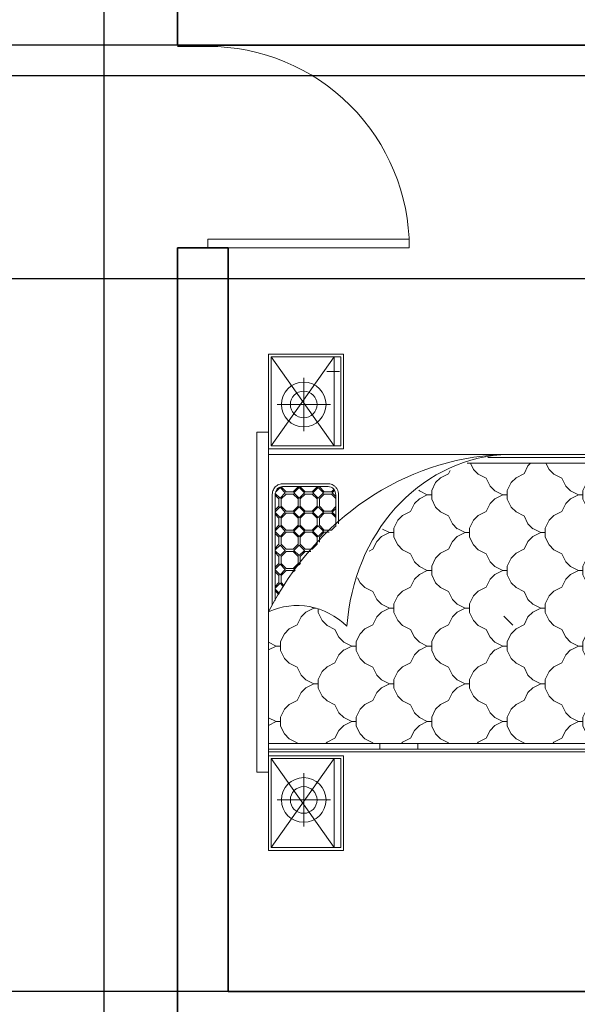
# Model space of a CAD drawing. Units: inches. Extents: x 1624 to 3956, y 1589 to 5028.
# Tile 4 of 16: x 1915 to 2014, y 2075 to 2250. Entities that reach past the tile are written whole.
import ezdxf

# ---------------------------------------------------------------- set-up
doc = ezdxf.new("R2010")
doc.units = ezdxf.units.IN
for name, color, linetype, lineweight in [('A-ANNO-DIMS', 2, 'Continuous', 13), ('A-DOOR', 3, 'Continuous', 18), ('A-FURN', 8, 'Continuous', 18), ('A-WALL', 7, 'Continuous', 35)]:
    doc.layers.add(name, color=color, linetype=linetype, lineweight=lineweight)
doc.styles.get("Standard").update_dxf_attribs({"font": 'arial.ttf'})
doc.dimstyles.new('Copy of ISO-25', dxfattribs={"dimtxt": 2.5, "dimasz": 2.5, "dimexe": 1.25, "dimexo": 0.625, "dimtad": 1, "dimdec": 1, "dimlunit": 4, "dimtxsty": 'Standard', "dimcen": 2.5, "dimadec": 0, "dimazin": 0, "dimtfac": 1, "dimtdec": 1, "dimtmove": 0, "dimatfit": 3, "dimfxl": 1, "dimarcsym": 0})

# ---------------------------------------------------------------- blocks, each defined once
blk = doc.blocks.new('*U5')
for p, q in [((0, 0), (0, 6)), ((40, 0), (40, 6))]:
    blk.add_line(p, q)
blk.add_lwpolyline([(0, 0), (0, -40), (1.75, -40), (1.75, 0)], close=True)
blk.add_arc((0, 0), 40, 270, 0)
blk = doc.blocks.new('A$C029D5C69')
for p, q in [((0.4164, 2.0693), (0.4164, 2.0066)), ((2.2315, 2.0693), (0.4164, 2.0693)), ((2.2315, 2.0066), (2.2315, 2.0693)), ((0, 1.606), (0, 2.0066)), ((0, 2.0066), (0.505, 2.0066)), ((0.4164, 2.0066), (2.2315, 2.0066)), ((0.505, 2.0066), (0.505, 1.606)), ((0.5252, 0.0351), (0.5252, 2.0066)), ((0.5403, 0.0502), (0.5403, 2.0066)), ((0.5706, 0.0805), (0.5706, 2.0066)), ((0.6869, 1.966), (0.6666, 2.0066)), ((0.7072, 2.0066), (0.6869, 1.966)), ((1.0902, 1.966), (1.0699, 2.0066)), ((1.1106, 2.0066), (1.0902, 1.966)), ((2.1114, 2.0087), (2.1114, 0.0351)), ((2.6479, 2.0066), (2.1429, 2.0066)), ((2.1429, 2.0066), (2.1429, 1.606)), ((2.6479, 1.606), (2.6479, 2.0066)), ((0.0151, 1.6211), (0.0151, 1.9915)), ((0.0151, 1.9915), (0.4899, 1.9915)), ((0.2689, 1.9609), (0.2689, 1.6764)), ((0.4899, 1.9915), (0.4899, 1.6211)), ((0.6869, 1.9425), (0.6869, 1.966)), ((0.6869, 1.9425), (0.6869, 1.966)), ((1.0902, 1.9425), (1.0902, 1.966)), ((1.0902, 1.9425), (1.0902, 1.966)), ((1.8954, 1.9865), (1.3081, 1.9865)), ((1.8954, 1.9713), (1.3339, 1.9713)), ((1.3849, 1.9713), (1.3656, 1.952)), ((1.3945, 1.9713), (1.3714, 1.9483)), ((1.4249, 1.945), (1.3986, 1.9713)), ((1.4249, 1.945), (1.4059, 1.926)), ((1.4288, 1.9507), (1.4081, 1.9713)), ((1.4476, 1.9507), (1.4288, 1.9507)), ((1.4476, 1.9507), (1.4664, 1.9507)), ((1.487, 1.9713), (1.4664, 1.9507)), ((1.4966, 1.9713), (1.4703, 1.945)), ((1.4986, 1.9167), (1.4703, 1.945)), ((1.527, 1.945), (1.4986, 1.9167)), ((1.527, 1.945), (1.5007, 1.9713)), ((1.5309, 1.9507), (1.5102, 1.9713)), ((1.5497, 1.9507), (1.5309, 1.9507)), ((1.5497, 1.9507), (1.5685, 1.9507)), ((1.5891, 1.9713), (1.5685, 1.9507)), ((1.5987, 1.9713), (1.5724, 1.945)), ((1.6007, 1.9167), (1.5724, 1.945)), ((1.6291, 1.945), (1.6007, 1.9167)), ((1.6291, 1.945), (1.6028, 1.9713)), ((1.633, 1.9507), (1.6123, 1.9713)), ((1.6518, 1.9507), (1.633, 1.9507)), ((1.6518, 1.9507), (1.6706, 1.9507)), ((1.6912, 1.9713), (1.6706, 1.9507)), ((1.7008, 1.9713), (1.6745, 1.945)), ((1.7028, 1.9167), (1.6745, 1.945)), ((1.7312, 1.945), (1.7028, 1.9167)), ((1.7312, 1.945), (1.7049, 1.9713)), ((1.7351, 1.9507), (1.7144, 1.9713)), ((1.7539, 1.9507), (1.7351, 1.9507)), ((1.7539, 1.9507), (1.7727, 1.9507)), ((1.7933, 1.9713), (1.7727, 1.9507)), ((1.8029, 1.9713), (1.7766, 1.945)), ((1.8049, 1.9167), (1.7766, 1.945)), ((1.8333, 1.945), (1.8049, 1.9167)), ((1.8333, 1.945), (1.807, 1.9713)), ((1.8372, 1.9507), (1.8165, 1.9713)), ((1.856, 1.9507), (1.8372, 1.9507)), ((1.856, 1.9507), (1.8748, 1.9507)), ((1.8954, 1.9713), (1.8748, 1.9507)), ((1.9043, 1.9707), (1.8787, 1.945)), ((1.907, 1.9167), (1.8787, 1.945)), ((1.9354, 1.945), (1.907, 1.9167)), ((1.9354, 1.945), (1.9114, 1.969)), ((2.6328, 1.9915), (2.158, 1.9915)), ((2.158, 1.9915), (2.158, 1.6211)), ((2.379, 1.9609), (2.379, 1.6764)), ((2.6328, 1.6211), (2.6328, 1.9915)), ((0.5955, 1.8958), (0.5743, 1.8534)), ((0.621, 1.9213), (0.5955, 1.8958)), ((0.6634, 1.9425), (0.621, 1.9213)), ((0.6634, 1.9425), (0.621, 1.9213)), ((0.6869, 1.9425), (0.6634, 1.9425)), ((0.6869, 1.9425), (0.7104, 1.9425)), ((0.7528, 1.9213), (0.7104, 1.9425)), ((0.7528, 1.9213), (0.7104, 1.9425)), ((0.7783, 1.8958), (0.7528, 1.9213)), ((0.7995, 1.8534), (0.7783, 1.8958)), ((0.9989, 1.8958), (0.9777, 1.8534)), ((1.0243, 1.9213), (0.9988, 1.8958)), ((1.0668, 1.9425), (1.0244, 1.9213)), ((1.0668, 1.9425), (1.0244, 1.9213)), ((1.0902, 1.9425), (1.0668, 1.9425)), ((1.0902, 1.9425), (1.1137, 1.9425)), ((1.1561, 1.9213), (1.1137, 1.9425)), ((1.1561, 1.9213), (1.1137, 1.9425)), ((1.1816, 1.8958), (1.1561, 1.9213)), ((1.2028, 1.8534), (1.1816, 1.8958)), ((1.4288, 1.9394), (1.4116, 1.9222)), ((1.4288, 1.9393), (1.4476, 1.9393)), ((1.4664, 1.9393), (1.4476, 1.9393)), ((1.493, 1.9128), (1.4664, 1.9394)), ((1.493, 1.8752), (1.493, 1.9128)), ((1.5309, 1.9394), (1.5043, 1.9128)), ((1.5043, 1.8752), (1.5043, 1.9128)), ((1.5309, 1.9393), (1.5497, 1.9393)), ((1.5685, 1.9393), (1.5497, 1.9393)), ((1.595, 1.9128), (1.5685, 1.9394)), ((1.595, 1.8752), (1.595, 1.9128)), ((1.633, 1.9394), (1.6064, 1.9128)), ((1.6064, 1.8752), (1.6064, 1.9128)), ((1.633, 1.9393), (1.6518, 1.9393)), ((1.6706, 1.9393), (1.6518, 1.9393)), ((1.6971, 1.9128), (1.6706, 1.9394)), ((1.6971, 1.8752), (1.6971, 1.9128)), ((1.7351, 1.9394), (1.7085, 1.9128)), ((1.7085, 1.8752), (1.7085, 1.9128)), ((1.7351, 1.9393), (1.7539, 1.9393)), ((1.7727, 1.9393), (1.7539, 1.9393)), ((1.7992, 1.9128), (1.7727, 1.9394)), ((1.7992, 1.8752), (1.7992, 1.9128)), ((1.8372, 1.9394), (1.8106, 1.9128)), ((1.8106, 1.8752), (1.8106, 1.9128)), ((1.8372, 1.9393), (1.856, 1.9393)), ((1.8748, 1.9393), (1.856, 1.9393)), ((1.9013, 1.9128), (1.8748, 1.9394)), ((1.9013, 1.8752), (1.9013, 1.9128)), ((1.9393, 1.9394), (1.9127, 1.9128)), ((1.9127, 1.8752), (1.9127, 1.9128)), ((1.9393, 1.9393), (1.9404, 1.9393)), ((1.9414, 1.688), (1.9414, 1.931)), ((1.9565, 1.688), (1.9565, 1.931)), ((0.5743, 1.8534), (0.5706, 1.8515)), ((0.5743, 1.8534), (0.5706, 1.8515)), ((0.8419, 1.8322), (0.7995, 1.8534)), ((0.8419, 1.8322), (0.7995, 1.8534)), ((0.9777, 1.8534), (0.9353, 1.8322)), ((0.9777, 1.8534), (0.9353, 1.8322)), ((1.2452, 1.8322), (1.2028, 1.8534)), ((1.2452, 1.8322), (1.2028, 1.8534)), ((1.493, 1.8752), (1.4867, 1.869)), ((1.4986, 1.8713), (1.4922, 1.8648)), ((1.527, 1.8429), (1.4986, 1.8713)), ((1.5309, 1.8486), (1.5043, 1.8752)), ((1.527, 1.8429), (1.5242, 1.8401)), ((1.5497, 1.8486), (1.5309, 1.8486)), ((1.5497, 1.8486), (1.5685, 1.8486)), ((1.595, 1.8752), (1.5685, 1.8486)), ((1.6007, 1.8713), (1.5724, 1.8429)), ((1.6007, 1.8146), (1.5724, 1.8429)), ((1.6291, 1.8429), (1.6007, 1.8713)), ((1.6291, 1.8429), (1.6007, 1.8146)), ((1.633, 1.8486), (1.6064, 1.8752)), ((1.6518, 1.8486), (1.633, 1.8486)), ((1.6518, 1.8486), (1.6706, 1.8486)), ((1.6971, 1.8752), (1.6706, 1.8486)), ((1.7028, 1.8713), (1.6745, 1.8429)), ((1.7028, 1.8146), (1.6745, 1.8429)), ((1.7312, 1.8429), (1.7028, 1.8713)), ((1.7312, 1.8429), (1.7028, 1.8146)), ((1.7351, 1.8486), (1.7085, 1.8752)), ((1.7539, 1.8486), (1.7351, 1.8486)), ((1.7539, 1.8486), (1.7727, 1.8486)), ((1.7992, 1.8752), (1.7727, 1.8486)), ((1.8049, 1.8713), (1.7766, 1.8429)), ((1.8049, 1.8146), (1.7766, 1.8429)), ((1.8333, 1.8429), (1.8049, 1.8713)), ((1.8333, 1.8429), (1.8049, 1.8146)), ((1.8372, 1.8486), (1.8106, 1.8752)), ((1.856, 1.8486), (1.8372, 1.8486)), ((1.856, 1.8486), (1.8748, 1.8486)), ((1.9013, 1.8752), (1.8748, 1.8486)), ((1.907, 1.8713), (1.8787, 1.8429)), ((1.907, 1.8146), (1.8787, 1.8429)), ((1.9354, 1.8429), (1.907, 1.8713)), ((1.9354, 1.8429), (1.907, 1.8146)), ((1.9393, 1.8486), (1.9127, 1.8752)), ((1.9414, 1.8486), (1.9393, 1.8486)), ((0.1267, 1.8186), (0.4111, 1.8186)), ((0.8674, 1.8067), (0.8419, 1.8322)), ((0.8886, 1.7643), (0.8674, 1.8067)), ((0.9098, 1.8067), (0.8886, 1.7643)), ((0.9352, 1.8322), (0.9097, 1.8067)), ((1.2707, 1.8067), (1.2452, 1.8322)), ((1.2919, 1.7643), (1.2707, 1.8067)), ((1.5309, 1.8373), (1.5295, 1.8359)), ((1.5309, 1.8373), (1.5497, 1.8373)), ((1.5685, 1.8373), (1.5497, 1.8373)), ((1.595, 1.8107), (1.5685, 1.8373)), ((1.595, 1.7806), (1.595, 1.8107)), ((1.633, 1.8373), (1.6064, 1.8107)), ((1.6064, 1.7731), (1.6064, 1.8107)), ((1.633, 1.8373), (1.6518, 1.8373)), ((1.6706, 1.8373), (1.6518, 1.8373)), ((1.6971, 1.8107), (1.6706, 1.8373)), ((1.6971, 1.7731), (1.6971, 1.8107)), ((1.7351, 1.8373), (1.7085, 1.8107)), ((1.7085, 1.7731), (1.7085, 1.8107)), ((1.7351, 1.8373), (1.7539, 1.8373)), ((1.7727, 1.8373), (1.7539, 1.8373)), ((1.7992, 1.8107), (1.7727, 1.8373)), ((1.7992, 1.7731), (1.7992, 1.8107)), ((1.8372, 1.8373), (1.8106, 1.8107)), ((1.8106, 1.7731), (1.8106, 1.8107)), ((1.8372, 1.8373), (1.856, 1.8373)), ((1.8748, 1.8373), (1.856, 1.8373)), ((1.9013, 1.8107), (1.8748, 1.8373)), ((1.9013, 1.7731), (1.9013, 1.8107)), ((1.9393, 1.8373), (1.9127, 1.8107)), ((1.9127, 1.7731), (1.9127, 1.8107)), ((1.9393, 1.8373), (1.9414, 1.8373)), ((2.2367, 1.8186), (2.5212, 1.8186)), ((0.8651, 1.7408), (0.8227, 1.7196)), ((0.8651, 1.7408), (0.8227, 1.7196)), ((0.912, 1.7408), (0.8651, 1.7408)), ((0.8886, 1.7408), (0.8886, 1.7643)), ((0.9544, 1.7196), (0.912, 1.7408)), ((0.9544, 1.7196), (0.912, 1.7408)), ((1.2684, 1.7408), (1.226, 1.7196)), ((1.2684, 1.7408), (1.226, 1.7196)), ((1.2885, 1.7408), (1.2684, 1.7408)), ((1.2981, 1.7768), (1.2919, 1.7643)), ((1.2919, 1.7519), (1.2919, 1.7643)), ((1.633, 1.7465), (1.6064, 1.7731)), ((1.6518, 1.7465), (1.633, 1.7465)), ((1.6443, 1.7352), (1.6518, 1.7352)), ((1.6518, 1.7465), (1.6706, 1.7465)), ((1.6706, 1.7352), (1.6518, 1.7352)), ((1.6971, 1.7731), (1.6706, 1.7465)), ((1.6971, 1.7086), (1.6706, 1.7352)), ((1.7028, 1.7692), (1.6745, 1.7408)), ((1.7028, 1.7125), (1.6745, 1.7408)), ((1.7312, 1.7408), (1.7028, 1.7692)), ((1.7312, 1.7408), (1.7028, 1.7125)), ((1.7351, 1.7465), (1.7085, 1.7731)), ((1.7351, 1.7352), (1.7085, 1.7086)), ((1.7539, 1.7465), (1.7351, 1.7465)), ((1.7351, 1.7352), (1.7539, 1.7352)), ((1.7539, 1.7465), (1.7727, 1.7465)), ((1.7727, 1.7352), (1.7539, 1.7352)), ((1.7992, 1.7731), (1.7727, 1.7465)), ((1.7992, 1.7086), (1.7727, 1.7352)), ((1.8049, 1.7692), (1.7766, 1.7408)), ((1.8049, 1.7125), (1.7766, 1.7408)), ((1.8333, 1.7408), (1.8049, 1.7692)), ((1.8333, 1.7408), (1.8049, 1.7125)), ((1.8372, 1.7465), (1.8106, 1.7731)), ((1.8372, 1.7352), (1.8106, 1.7086)), ((1.856, 1.7465), (1.8372, 1.7465)), ((1.8372, 1.7352), (1.856, 1.7352)), ((1.856, 1.7465), (1.8748, 1.7465)), ((1.8748, 1.7352), (1.856, 1.7352)), ((1.9013, 1.7731), (1.8748, 1.7465)), ((1.9013, 1.7086), (1.8748, 1.7352)), ((1.907, 1.7692), (1.8787, 1.7408)), ((1.907, 1.7125), (1.8787, 1.7408)), ((1.9354, 1.7408), (1.907, 1.7692)), ((1.9354, 1.7408), (1.907, 1.7125)), ((1.9393, 1.7465), (1.9127, 1.7731)), ((1.9393, 1.7352), (1.9127, 1.7086)), ((1.9414, 1.7465), (1.9393, 1.7465)), ((1.9393, 1.7352), (1.9414, 1.7352)), ((0.5766, 1.6941), (0.5706, 1.7002)), ((0.5978, 1.6517), (0.5766, 1.6941)), ((0.7972, 1.6941), (0.776, 1.6517)), ((0.8227, 1.7196), (0.7972, 1.6941)), ((0.98, 1.6941), (0.9545, 1.7196)), ((1.0011, 1.6517), (0.9799, 1.6941)), ((1.2005, 1.6941), (1.1793, 1.6517)), ((1.226, 1.7196), (1.2005, 1.6941)), ((1.6971, 1.682), (1.6971, 1.7086)), ((1.7085, 1.671), (1.7085, 1.7086)), ((1.7992, 1.671), (1.7992, 1.7086)), ((1.8106, 1.671), (1.8106, 1.7086)), ((1.9013, 1.671), (1.9013, 1.7086)), ((1.9127, 1.671), (1.9127, 1.7086)), ((2.5551, 1.6275), (2.5551, 1.696)), ((0.6402, 1.6305), (0.5978, 1.6517)), ((0.6402, 1.6305), (0.5978, 1.6517)), ((0.6657, 1.605), (0.6402, 1.6305)), ((0.7336, 1.6305), (0.7081, 1.605)), ((0.776, 1.6517), (0.7336, 1.6305)), ((0.776, 1.6517), (0.7336, 1.6305)), ((1.0435, 1.6305), (1.0011, 1.6517)), ((1.0435, 1.6305), (1.0011, 1.6517)), ((1.0691, 1.605), (1.0436, 1.6305)), ((1.1369, 1.6305), (1.1114, 1.605)), ((1.1793, 1.6517), (1.1369, 1.6305)), ((1.1793, 1.6517), (1.1369, 1.6305)), ((1.7318, 1.6477), (1.7085, 1.671)), ((1.8961, 1.6477), (1.7289, 1.6477)), ((1.8961, 1.6325), (1.7422, 1.6325)), ((1.7992, 1.671), (1.7759, 1.6477)), ((1.8049, 1.6671), (1.7855, 1.6477)), ((1.8244, 1.6477), (1.8049, 1.6671)), ((1.8339, 1.6477), (1.8106, 1.671)), ((1.9013, 1.671), (1.878, 1.6477)), ((1.907, 1.6671), (1.8876, 1.6477)), ((1.9202, 1.6539), (1.907, 1.6671)), ((1.926, 1.6577), (1.9127, 1.671)), ((0.505, 1.606), (0, 1.606)), ((0.4899, 1.6211), (0.0151, 1.6211)), ((0.6869, 1.5626), (0.6657, 1.605)), ((0.7081, 1.605), (0.6869, 1.5626)), ((1.0902, 1.5626), (1.069, 1.605)), ((1.1114, 1.605), (1.0902, 1.5626)), ((2.1429, 1.606), (2.6479, 1.606)), ((2.158, 1.6211), (2.6328, 1.6211)), ((0.6634, 1.5391), (0.621, 1.5179)), ((0.6634, 1.5391), (0.621, 1.5179)), ((0.6869, 1.5392), (0.6634, 1.5392)), ((0.6869, 1.5392), (0.6869, 1.5626)), ((0.6869, 1.5392), (0.6869, 1.5626)), ((0.6869, 1.5392), (0.7104, 1.5392)), ((0.7528, 1.5179), (0.7104, 1.5391)), ((0.7528, 1.5179), (0.7104, 1.5391)), ((1.0668, 1.5391), (1.0244, 1.5179)), ((1.0668, 1.5391), (1.0244, 1.5179)), ((1.0902, 1.5392), (1.0668, 1.5392)), ((1.0902, 1.5392), (1.0902, 1.5626)), ((1.0902, 1.5392), (1.0902, 1.5626)), ((1.0902, 1.5392), (1.1137, 1.5392)), ((1.1561, 1.5179), (1.1137, 1.5391)), ((1.1561, 1.5179), (1.1137, 1.5391)), ((1.4534, 1.5308), (1.4277, 1.5179)), ((1.4534, 1.5308), (1.4277, 1.5179)), ((0.5955, 1.4925), (0.5743, 1.4501)), ((0.621, 1.5179), (0.5955, 1.4924)), ((0.7783, 1.4924), (0.7528, 1.5179)), ((0.7995, 1.4501), (0.7783, 1.4925)), ((0.9989, 1.4925), (0.9777, 1.4501)), ((1.0243, 1.5179), (0.9988, 1.4924)), ((1.1816, 1.4924), (1.1561, 1.5179)), ((1.2028, 1.4501), (1.1816, 1.4925)), ((1.4022, 1.4925), (1.381, 1.4501)), ((1.4277, 1.5179), (1.4022, 1.4924)), ((0.5743, 1.45), (0.5706, 1.4481)), ((0.5743, 1.45), (0.5706, 1.4481)), ((0.8419, 1.4288), (0.7995, 1.45)), ((0.8419, 1.4288), (0.7995, 1.45)), ((0.8674, 1.4033), (0.8419, 1.4288)), ((0.9352, 1.4288), (0.9097, 1.4033)), ((0.9777, 1.45), (0.9353, 1.4288)), ((0.9777, 1.45), (0.9353, 1.4288)), ((1.2452, 1.4288), (1.2028, 1.45)), ((1.2452, 1.4288), (1.2028, 1.45)), ((1.2707, 1.4033), (1.2452, 1.4288)), ((1.3386, 1.4288), (1.3131, 1.4033)), ((1.381, 1.45), (1.3386, 1.4288)), ((1.381, 1.45), (1.3386, 1.4288)), ((1.6062, 1.4501), (1.5966, 1.4692)), ((1.6486, 1.4288), (1.6062, 1.45)), ((1.6486, 1.4288), (1.6062, 1.45)), ((1.6741, 1.4033), (1.6486, 1.4288)), ((0.5403, 1.4117), (0.5706, 1.4117)), ((0.8886, 1.361), (0.8674, 1.4034)), ((0.9098, 1.4034), (0.8886, 1.361)), ((1.2919, 1.361), (1.2707, 1.4034)), ((1.3131, 1.4034), (1.2919, 1.361)), ((1.6953, 1.361), (1.6741, 1.4034)), ((1.714, 1.3984), (1.6953, 1.361)), ((0.8227, 1.3163), (0.7972, 1.2908)), ((0.8651, 1.3374), (0.8227, 1.3162)), ((0.8651, 1.3374), (0.8227, 1.3162)), ((0.912, 1.3375), (0.8651, 1.3375)), ((0.8886, 1.3375), (0.8886, 1.3609)), ((0.9544, 1.3162), (0.912, 1.3374)), ((0.9544, 1.3162), (0.912, 1.3374)), ((0.98, 1.2908), (0.9545, 1.3163)), ((1.226, 1.3163), (1.2005, 1.2908)), ((1.2684, 1.3374), (1.226, 1.3162)), ((1.2684, 1.3374), (1.226, 1.3162)), ((1.3154, 1.3375), (1.2684, 1.3375)), ((1.2919, 1.3375), (1.2919, 1.3609)), ((1.3578, 1.3162), (1.3154, 1.3374)), ((1.3578, 1.3162), (1.3154, 1.3374)), ((1.3833, 1.2908), (1.3578, 1.3163)), ((1.6294, 1.3163), (1.6039, 1.2908)), ((1.6718, 1.3374), (1.6294, 1.3162)), ((1.6718, 1.3374), (1.6294, 1.3162)), ((1.7187, 1.3375), (1.6718, 1.3375)), ((1.6953, 1.3375), (1.6953, 1.3609)), ((1.7611, 1.3162), (1.7187, 1.3374)), ((1.7611, 1.3162), (1.7187, 1.3374)), ((1.7867, 1.2908), (1.7611, 1.3163)), ((0.5766, 1.2908), (0.5706, 1.2968)), ((0.5978, 1.2484), (0.5766, 1.2908)), ((0.7972, 1.2908), (0.776, 1.2484)), ((1.0011, 1.2484), (0.9799, 1.2908)), ((1.2005, 1.2908), (1.1793, 1.2484)), ((1.4045, 1.2484), (1.3833, 1.2908)), ((1.6039, 1.2908), (1.5827, 1.2484)), ((1.8078, 1.2484), (1.7866, 1.2908)), ((0.5403, 1.21), (0.5706, 1.21)), ((0.6402, 1.2271), (0.5978, 1.2483)), ((0.6402, 1.2271), (0.5978, 1.2483)), ((0.6657, 1.2017), (0.6402, 1.2272)), ((0.7336, 1.2272), (0.7081, 1.2017)), ((0.776, 1.2483), (0.7336, 1.2271)), ((0.776, 1.2483), (0.7336, 1.2271)), ((1.0435, 1.2271), (1.0011, 1.2483)), ((1.0435, 1.2271), (1.0011, 1.2483)), ((1.0691, 1.2017), (1.0436, 1.2272)), ((1.1369, 1.2272), (1.1114, 1.2017)), ((1.1793, 1.2483), (1.1369, 1.2271)), ((1.1793, 1.2483), (1.1369, 1.2271)), ((1.4469, 1.2271), (1.4045, 1.2483)), ((1.4469, 1.2271), (1.4045, 1.2483)), ((1.4724, 1.2017), (1.4469, 1.2272)), ((1.5403, 1.2272), (1.5148, 1.2017)), ((1.5827, 1.2483), (1.5403, 1.2271)), ((1.5827, 1.2483), (1.5403, 1.2271)), ((1.8502, 1.2271), (1.8078, 1.2483)), ((1.8502, 1.2271), (1.8078, 1.2483)), ((1.8758, 1.2017), (1.8503, 1.2272)), ((0.6869, 1.1593), (0.6657, 1.2017)), ((0.7081, 1.2017), (0.6869, 1.1593)), ((0.6869, 1.1358), (0.6869, 1.1593)), ((0.6869, 1.1358), (0.6869, 1.1593)), ((1.0902, 1.1593), (1.069, 1.2017)), ((1.1114, 1.2017), (1.0902, 1.1593)), ((1.0902, 1.1358), (1.0902, 1.1593)), ((1.0902, 1.1358), (1.0902, 1.1593)), ((1.4936, 1.1593), (1.4724, 1.2017)), ((1.5148, 1.2017), (1.4936, 1.1593)), ((1.4936, 1.1358), (1.4936, 1.1593)), ((1.4936, 1.1358), (1.4936, 1.1593)), ((1.8969, 1.1593), (1.8757, 1.2017)), ((1.9181, 1.2017), (1.8969, 1.1593)), ((1.8969, 1.1358), (1.8969, 1.1593)), ((1.8969, 1.1358), (1.8969, 1.1593)), ((1.9215, 1.2051), (1.9181, 1.2017)), ((0.621, 1.1146), (0.5955, 1.0891)), ((0.6634, 1.1358), (0.621, 1.1146)), ((0.6634, 1.1358), (0.621, 1.1146)), ((0.6869, 1.1358), (0.6634, 1.1358)), ((0.6869, 1.1358), (0.7104, 1.1358)), ((0.7528, 1.1146), (0.7104, 1.1358)), ((0.7528, 1.1146), (0.7104, 1.1358)), ((0.7783, 1.0891), (0.7528, 1.1146)), ((1.0243, 1.1146), (0.9988, 1.0891)), ((1.0668, 1.1358), (1.0244, 1.1146)), ((1.0668, 1.1358), (1.0244, 1.1146)), ((1.0902, 1.1358), (1.0668, 1.1358)), ((1.0902, 1.1358), (1.1137, 1.1358)), ((1.1561, 1.1146), (1.1137, 1.1358)), ((1.1561, 1.1146), (1.1137, 1.1358)), ((1.1816, 1.0891), (1.1561, 1.1146)), ((1.4277, 1.1146), (1.4022, 1.0891)), ((1.4701, 1.1358), (1.4277, 1.1146)), ((1.4701, 1.1358), (1.4277, 1.1146)), ((1.4936, 1.1358), (1.4701, 1.1358)), ((1.4936, 1.1358), (1.5171, 1.1358)), ((1.5595, 1.1146), (1.5171, 1.1358)), ((1.5595, 1.1146), (1.5171, 1.1358)), ((1.585, 1.0891), (1.5595, 1.1146)), ((1.831, 1.1146), (1.8055, 1.0891)), ((1.8735, 1.1358), (1.8311, 1.1146)), ((1.8735, 1.1358), (1.8311, 1.1146)), ((1.8969, 1.1358), (1.8735, 1.1358)), ((1.8969, 1.1358), (1.9204, 1.1358)), ((1.9628, 1.1146), (1.9204, 1.1358)), ((1.9628, 1.1146), (1.9204, 1.1358)), ((1.9883, 1.0891), (1.9628, 1.1146)), ((0.5955, 1.0891), (0.5743, 1.0467)), ((0.7995, 1.0467), (0.7783, 1.0891)), ((0.9989, 1.0891), (0.9777, 1.0467)), ((1.2028, 1.0467), (1.1816, 1.0891)), ((1.4022, 1.0891), (1.381, 1.0467)), ((1.6062, 1.0467), (1.585, 1.0891)), ((1.8056, 1.0891), (1.7844, 1.0467)), ((2.0095, 1.0467), (1.9883, 1.0891)), ((0.5743, 1.0467), (0.5706, 1.0448)), ((0.5743, 1.0467), (0.5706, 1.0448)), ((0.8419, 1.0255), (0.7995, 1.0467)), ((0.8419, 1.0255), (0.7995, 1.0467)), ((0.8674, 1), (0.8419, 1.0255)), ((0.8886, 0.9576), (0.8674, 1)), ((0.9098, 1), (0.8886, 0.9576)), ((0.9352, 1.0255), (0.9097, 1)), ((0.9777, 1.0467), (0.9353, 1.0255)), ((0.9777, 1.0467), (0.9353, 1.0255)), ((1.2452, 1.0255), (1.2028, 1.0467)), ((1.2452, 1.0255), (1.2028, 1.0467)), ((1.2707, 1), (1.2452, 1.0255)), ((1.2919, 0.9576), (1.2707, 1)), ((1.3131, 1), (1.2919, 0.9576)), ((1.3386, 1.0255), (1.3131, 1)), ((1.381, 1.0467), (1.3386, 1.0255)), ((1.381, 1.0467), (1.3386, 1.0255)), ((1.6486, 1.0255), (1.6062, 1.0467)), ((1.6486, 1.0255), (1.6062, 1.0467)), ((1.6741, 1), (1.6486, 1.0255)), ((1.6953, 0.9576), (1.6741, 1)), ((1.7165, 1), (1.6953, 0.9576)), ((1.7419, 1.0255), (1.7164, 1)), ((1.7844, 1.0467), (1.742, 1.0255)), ((1.7844, 1.0467), (1.742, 1.0255)), ((2.0276, 1.0376), (2.0095, 1.0467)), ((2.0276, 1.0376), (2.0095, 1.0467)), ((0.8886, 0.9341), (0.8886, 0.9576)), ((1.2919, 0.9341), (1.2919, 0.9576)), ((1.6953, 0.9341), (1.6953, 0.9576)), ((2.066, 0.9457), (2.066, 0.0805)), ((0.5766, 0.8874), (0.5706, 0.8935)), ((0.8227, 0.9129), (0.7972, 0.8874)), ((0.8651, 0.9341), (0.8227, 0.9129)), ((0.8651, 0.9341), (0.8227, 0.9129)), ((0.912, 0.9341), (0.8651, 0.9341)), ((0.9544, 0.9129), (0.912, 0.9341)), ((0.9544, 0.9129), (0.912, 0.9341)), ((0.98, 0.8874), (0.9545, 0.9129)), ((1.226, 0.9129), (1.2005, 0.8874)), ((1.2684, 0.9341), (1.226, 0.9129)), ((1.2684, 0.9341), (1.226, 0.9129)), ((1.3154, 0.9341), (1.2684, 0.9341)), ((1.3578, 0.9129), (1.3154, 0.9341)), ((1.3578, 0.9129), (1.3154, 0.9341)), ((1.3833, 0.8874), (1.3578, 0.9129)), ((1.6294, 0.9129), (1.6039, 0.8874)), ((1.6718, 0.9341), (1.6294, 0.9129)), ((1.6718, 0.9341), (1.6294, 0.9129)), ((1.7187, 0.9341), (1.6718, 0.9341)), ((1.7611, 0.9129), (1.7187, 0.9341)), ((1.7611, 0.9129), (1.7187, 0.9341)), ((1.7867, 0.8874), (1.7611, 0.9129)), ((2.0327, 0.9129), (2.0072, 0.8874)), ((2.066, 0.9295), (2.0327, 0.9129)), ((2.066, 0.9295), (2.0327, 0.9129)), ((0.5978, 0.845), (0.5766, 0.8874)), ((0.6402, 0.8238), (0.5978, 0.845)), ((0.6402, 0.8238), (0.5978, 0.845)), ((0.776, 0.845), (0.7336, 0.8238)), ((0.776, 0.845), (0.7336, 0.8238)), ((0.7972, 0.8874), (0.776, 0.845)), ((1.0011, 0.845), (0.9799, 0.8874)), ((1.0435, 0.8238), (1.0011, 0.845)), ((1.0435, 0.8238), (1.0011, 0.845)), ((1.1793, 0.845), (1.1369, 0.8238)), ((1.1793, 0.845), (1.1369, 0.8238)), ((1.2005, 0.8874), (1.1793, 0.845)), ((1.4045, 0.845), (1.3833, 0.8874)), ((1.4469, 0.8238), (1.4045, 0.845)), ((1.4469, 0.8238), (1.4045, 0.845)), ((1.5827, 0.845), (1.5403, 0.8238)), ((1.5827, 0.845), (1.5403, 0.8238)), ((1.6039, 0.8874), (1.5827, 0.845)), ((1.8078, 0.845), (1.7866, 0.8874)), ((1.8502, 0.8238), (1.8078, 0.845)), ((1.8502, 0.8238), (1.8078, 0.845)), ((1.986, 0.845), (1.9436, 0.8238)), ((1.986, 0.845), (1.9436, 0.8238)), ((2.0072, 0.8874), (1.986, 0.845)), ((0.6657, 0.7983), (0.6402, 0.8238)), ((0.6869, 0.7559), (0.6657, 0.7983)), ((0.7081, 0.7983), (0.6869, 0.7559)), ((0.7336, 0.8238), (0.7081, 0.7983)), ((1.0691, 0.7983), (1.0436, 0.8238)), ((1.0902, 0.7559), (1.069, 0.7983)), ((1.1114, 0.7983), (1.0902, 0.7559)), ((1.1369, 0.8238), (1.1114, 0.7983)), ((1.4724, 0.7983), (1.4469, 0.8238)), ((1.4936, 0.7559), (1.4724, 0.7983)), ((1.5148, 0.7983), (1.4936, 0.7559)), ((1.5403, 0.8238), (1.5148, 0.7983)), ((1.8758, 0.7983), (1.8503, 0.8238)), ((1.8969, 0.7559), (1.8757, 0.7983)), ((1.9181, 0.7983), (1.8969, 0.7559)), ((1.9436, 0.8238), (1.9181, 0.7983)), ((2.0962, 0.8369), (2.0962, 0.0502)), ((0.6869, 0.7325), (0.6869, 0.7559)), ((0.6869, 0.7325), (0.6869, 0.7559)), ((1.0902, 0.7325), (1.0902, 0.7559)), ((1.0902, 0.7325), (1.0902, 0.7559)), ((1.2024, 0.7028), (1.2503, 0.7507)), ((1.4936, 0.7325), (1.4936, 0.7559)), ((1.4936, 0.7325), (1.4936, 0.7559)), ((1.8969, 0.7325), (1.8969, 0.7559)), ((1.8969, 0.7325), (1.8969, 0.7559)), ((0.5955, 0.6858), (0.5743, 0.6434)), ((0.621, 0.7113), (0.5955, 0.6858)), ((0.6634, 0.7324), (0.621, 0.7112)), ((0.6634, 0.7324), (0.621, 0.7112)), ((0.6869, 0.7325), (0.6634, 0.7325)), ((0.6869, 0.7325), (0.7104, 0.7325)), ((0.7528, 0.7112), (0.7104, 0.7324)), ((0.7528, 0.7112), (0.7104, 0.7324)), ((0.7783, 0.6858), (0.7528, 0.7113)), ((0.7995, 0.6434), (0.7783, 0.6858)), ((0.9989, 0.6858), (0.9777, 0.6434)), ((1.0243, 0.7113), (0.9988, 0.6858)), ((1.0668, 0.7324), (1.0244, 0.7112)), ((1.0668, 0.7324), (1.0244, 0.7112)), ((1.0902, 0.7325), (1.0668, 0.7325)), ((1.0902, 0.7325), (1.1137, 0.7325)), ((1.1561, 0.7112), (1.1137, 0.7324)), ((1.1561, 0.7112), (1.1137, 0.7324)), ((1.1816, 0.6858), (1.1561, 0.7113)), ((1.2028, 0.6434), (1.1816, 0.6858)), ((1.4022, 0.6858), (1.381, 0.6434)), ((1.4277, 0.7113), (1.4022, 0.6858)), ((1.4701, 0.7324), (1.4277, 0.7112)), ((1.4701, 0.7324), (1.4277, 0.7112)), ((1.4936, 0.7325), (1.4701, 0.7325)), ((1.4936, 0.7325), (1.5171, 0.7325)), ((1.5595, 0.7112), (1.5171, 0.7324)), ((1.5595, 0.7112), (1.5171, 0.7324)), ((1.585, 0.6858), (1.5595, 0.7113)), ((1.6062, 0.6434), (1.585, 0.6858)), ((1.8056, 0.6858), (1.7844, 0.6434)), ((1.831, 0.7113), (1.8055, 0.6858)), ((1.8735, 0.7324), (1.8311, 0.7112)), ((1.8735, 0.7324), (1.8311, 0.7112)), ((1.8969, 0.7325), (1.8735, 0.7325)), ((1.8969, 0.7325), (1.9204, 0.7325)), ((1.9628, 0.7112), (1.9204, 0.7324)), ((1.9628, 0.7112), (1.9204, 0.7324)), ((1.9883, 0.6858), (1.9628, 0.7113)), ((2.0095, 0.6434), (1.9883, 0.6858)), ((0.5743, 0.6433), (0.5706, 0.6414)), ((0.5743, 0.6433), (0.5706, 0.6414)), ((0.8419, 0.6221), (0.7995, 0.6433)), ((0.8419, 0.6221), (0.7995, 0.6433)), ((0.9777, 0.6433), (0.9353, 0.6221)), ((0.9777, 0.6433), (0.9353, 0.6221)), ((1.2452, 0.6221), (1.2028, 0.6433)), ((1.2452, 0.6221), (1.2028, 0.6433)), ((1.381, 0.6433), (1.3386, 0.6221)), ((1.381, 0.6433), (1.3386, 0.6221)), ((1.6486, 0.6221), (1.6062, 0.6433)), ((1.6486, 0.6221), (1.6062, 0.6433)), ((1.7844, 0.6433), (1.742, 0.6221)), ((1.7844, 0.6433), (1.742, 0.6221)), ((2.0519, 0.6221), (2.0095, 0.6433)), ((2.0519, 0.6221), (2.0095, 0.6433)), ((0.8674, 0.5967), (0.8419, 0.6222)), ((0.8886, 0.5543), (0.8674, 0.5967)), ((0.9098, 0.5967), (0.8886, 0.5543)), ((0.9352, 0.6222), (0.9097, 0.5967)), ((1.2707, 0.5967), (1.2452, 0.6222)), ((1.2919, 0.5543), (1.2707, 0.5967)), ((1.3131, 0.5967), (1.2919, 0.5543)), ((1.3386, 0.6222), (1.3131, 0.5967)), ((1.6741, 0.5967), (1.6486, 0.6222)), ((1.6953, 0.5543), (1.6741, 0.5967)), ((1.7165, 0.5967), (1.6953, 0.5543)), ((1.7419, 0.6222), (1.7164, 0.5967)), ((2.066, 0.6081), (2.0519, 0.6222)), ((0.8651, 0.5308), (0.8227, 0.5096)), ((0.8651, 0.5308), (0.8227, 0.5096)), ((0.912, 0.5308), (0.8651, 0.5308)), ((0.8886, 0.5308), (0.8886, 0.5543)), ((0.9544, 0.5096), (0.912, 0.5308)), ((0.9544, 0.5096), (0.912, 0.5308)), ((1.2684, 0.5308), (1.226, 0.5096)), ((1.2684, 0.5308), (1.226, 0.5096)), ((1.3154, 0.5308), (1.2684, 0.5308)), ((1.2919, 0.5308), (1.2919, 0.5543)), ((1.3578, 0.5096), (1.3154, 0.5308)), ((1.3578, 0.5096), (1.3154, 0.5308)), ((1.6718, 0.5308), (1.6294, 0.5096)), ((1.6718, 0.5308), (1.6294, 0.5096)), ((1.7187, 0.5308), (1.6718, 0.5308)), ((1.6953, 0.5308), (1.6953, 0.5543)), ((1.7611, 0.5096), (1.7187, 0.5308)), ((1.7611, 0.5096), (1.7187, 0.5308)), ((2.066, 0.5262), (2.0327, 0.5096)), ((2.066, 0.5262), (2.0327, 0.5096)), ((0.5766, 0.4841), (0.5706, 0.4901)), ((0.5978, 0.4417), (0.5766, 0.4841)), ((0.7972, 0.4841), (0.776, 0.4417)), ((0.8227, 0.5096), (0.7972, 0.4841)), ((0.98, 0.4841), (0.9545, 0.5096)), ((1.0011, 0.4417), (0.9799, 0.4841)), ((1.2005, 0.4841), (1.1793, 0.4417)), ((1.226, 0.5096), (1.2005, 0.4841)), ((1.3833, 0.4841), (1.3578, 0.5096)), ((1.4045, 0.4417), (1.3833, 0.4841)), ((1.6039, 0.4841), (1.5827, 0.4417)), ((1.6294, 0.5096), (1.6039, 0.4841)), ((1.7867, 0.4841), (1.7611, 0.5096)), ((1.8078, 0.4417), (1.7866, 0.4841)), ((2.0072, 0.4841), (1.986, 0.4417)), ((2.0327, 0.5096), (2.0072, 0.4841)), ((0.6402, 0.4205), (0.5978, 0.4417)), ((0.6402, 0.4205), (0.5978, 0.4417)), ((0.6657, 0.395), (0.6402, 0.4205)), ((0.7336, 0.4205), (0.7081, 0.395)), ((0.776, 0.4417), (0.7336, 0.4205)), ((0.776, 0.4417), (0.7336, 0.4205)), ((1.0435, 0.4205), (1.0011, 0.4417)), ((1.0435, 0.4205), (1.0011, 0.4417)), ((1.0691, 0.395), (1.0436, 0.4205)), ((1.1369, 0.4205), (1.1114, 0.395)), ((1.1793, 0.4417), (1.1369, 0.4205)), ((1.1793, 0.4417), (1.1369, 0.4205)), ((1.4469, 0.4205), (1.4045, 0.4417)), ((1.4469, 0.4205), (1.4045, 0.4417)), ((1.4724, 0.395), (1.4469, 0.4205)), ((1.5403, 0.4205), (1.5148, 0.395)), ((1.5827, 0.4417), (1.5403, 0.4205)), ((1.5827, 0.4417), (1.5403, 0.4205)), ((1.8502, 0.4205), (1.8078, 0.4417)), ((1.8502, 0.4205), (1.8078, 0.4417)), ((1.8758, 0.395), (1.8503, 0.4205)), ((1.9436, 0.4205), (1.9181, 0.395)), ((1.986, 0.4417), (1.9436, 0.4205)), ((1.986, 0.4417), (1.9436, 0.4205)), ((0.6869, 0.3526), (0.6657, 0.395)), ((0.7081, 0.395), (0.6869, 0.3526)), ((1.0902, 0.3526), (1.069, 0.395)), ((1.1114, 0.395), (1.0902, 0.3526)), ((1.4936, 0.3526), (1.4724, 0.395)), ((1.5148, 0.395), (1.4936, 0.3526)), ((1.8969, 0.3526), (1.8757, 0.395)), ((1.9181, 0.395), (1.8969, 0.3526)), ((0.6634, 0.3291), (0.621, 0.3079)), ((0.6634, 0.3291), (0.621, 0.3079)), ((0.6869, 0.3291), (0.6634, 0.3291)), ((0.6869, 0.3291), (0.6869, 0.3526)), ((0.6869, 0.3291), (0.6869, 0.3526)), ((0.6869, 0.3291), (0.7104, 0.3291)), ((0.7528, 0.3079), (0.7104, 0.3291)), ((0.7528, 0.3079), (0.7104, 0.3291)), ((1.0668, 0.3291), (1.0244, 0.3079)), ((1.0668, 0.3291), (1.0244, 0.3079)), ((1.0902, 0.3291), (1.0668, 0.3291)), ((1.0902, 0.3291), (1.0902, 0.3526)), ((1.0902, 0.3291), (1.0902, 0.3526)), ((1.0902, 0.3291), (1.1137, 0.3291)), ((1.1561, 0.3079), (1.1137, 0.3291)), ((1.1561, 0.3079), (1.1137, 0.3291)), ((1.4701, 0.3291), (1.4277, 0.3079)), ((1.4701, 0.3291), (1.4277, 0.3079)), ((1.4936, 0.3291), (1.4701, 0.3291)), ((1.4936, 0.3291), (1.4936, 0.3526)), ((1.4936, 0.3291), (1.4936, 0.3526)), ((1.4936, 0.3291), (1.5171, 0.3291)), ((1.5595, 0.3079), (1.5171, 0.3291)), ((1.5595, 0.3079), (1.5171, 0.3291)), ((1.8735, 0.3291), (1.8311, 0.3079)), ((1.8735, 0.3291), (1.8311, 0.3079)), ((1.8969, 0.3291), (1.8735, 0.3291)), ((1.8969, 0.3291), (1.8969, 0.3526)), ((1.8969, 0.3291), (1.8969, 0.3526)), ((1.8969, 0.3291), (1.9204, 0.3291)), ((1.9628, 0.3079), (1.9204, 0.3291)), ((1.9628, 0.3079), (1.9204, 0.3291)), ((0.5955, 0.2824), (0.5743, 0.24)), ((0.621, 0.3079), (0.5955, 0.2824)), ((0.7783, 0.2824), (0.7528, 0.3079)), ((0.7995, 0.24), (0.7783, 0.2824)), ((0.9989, 0.2824), (0.9777, 0.24)), ((1.0243, 0.3079), (0.9988, 0.2824)), ((1.1816, 0.2824), (1.1561, 0.3079)), ((1.2028, 0.24), (1.1816, 0.2824)), ((1.4022, 0.2824), (1.381, 0.24)), ((1.4277, 0.3079), (1.4022, 0.2824)), ((1.585, 0.2824), (1.5595, 0.3079)), ((1.6062, 0.24), (1.585, 0.2824)), ((1.8056, 0.2824), (1.7844, 0.24)), ((1.831, 0.3079), (1.8055, 0.2824)), ((1.9883, 0.2824), (1.9628, 0.3079)), ((2.0095, 0.24), (1.9883, 0.2824)), ((0.5743, 0.24), (0.5706, 0.2381)), ((0.5743, 0.24), (0.5706, 0.2381)), ((0.8419, 0.2188), (0.7995, 0.24)), ((0.8419, 0.2188), (0.7995, 0.24)), ((0.8674, 0.1933), (0.8419, 0.2188)), ((0.9352, 0.2188), (0.9097, 0.1933)), ((0.9777, 0.24), (0.9353, 0.2188)), ((0.9777, 0.24), (0.9353, 0.2188)), ((1.2452, 0.2188), (1.2028, 0.24)), ((1.2452, 0.2188), (1.2028, 0.24)), ((1.2707, 0.1933), (1.2452, 0.2188)), ((1.3386, 0.2188), (1.3131, 0.1933)), ((1.381, 0.24), (1.3386, 0.2188)), ((1.381, 0.24), (1.3386, 0.2188)), ((1.6486, 0.2188), (1.6062, 0.24)), ((1.6486, 0.2188), (1.6062, 0.24)), ((1.6741, 0.1933), (1.6486, 0.2188)), ((1.7419, 0.2188), (1.7164, 0.1933)), ((1.7844, 0.24), (1.742, 0.2188)), ((1.7844, 0.24), (1.742, 0.2188)), ((2.0519, 0.2188), (2.0095, 0.24)), ((2.0519, 0.2188), (2.0095, 0.24)), ((2.066, 0.2047), (2.0519, 0.2188)), ((0.8886, 0.1509), (0.8674, 0.1933)), ((0.9098, 0.1933), (0.8886, 0.1509)), ((1.2919, 0.1509), (1.2707, 0.1933)), ((1.3131, 0.1933), (1.2919, 0.1509)), ((1.6953, 0.1509), (1.6741, 0.1933)), ((1.7165, 0.1933), (1.6953, 0.1509)), ((0.8227, 0.1062), (0.7972, 0.0807)), ((0.8651, 0.1274), (0.8227, 0.1062)), ((0.8651, 0.1274), (0.8227, 0.1062)), ((0.912, 0.1275), (0.8651, 0.1275)), ((0.8886, 0.1275), (0.8886, 0.1509)), ((0.9544, 0.1062), (0.912, 0.1274)), ((0.9544, 0.1062), (0.912, 0.1274)), ((0.98, 0.0807), (0.9545, 0.1062)), ((1.226, 0.1062), (1.2005, 0.0807)), ((1.2684, 0.1274), (1.226, 0.1062)), ((1.2684, 0.1274), (1.226, 0.1062)), ((1.3154, 0.1275), (1.2684, 0.1275)), ((1.2919, 0.1275), (1.2919, 0.1509)), ((1.3578, 0.1062), (1.3154, 0.1274)), ((1.3578, 0.1062), (1.3154, 0.1274)), ((1.3833, 0.0807), (1.3578, 0.1062)), ((1.6294, 0.1062), (1.6039, 0.0807)), ((1.6718, 0.1274), (1.6294, 0.1062)), ((1.6718, 0.1274), (1.6294, 0.1062)), ((1.7187, 0.1275), (1.6718, 0.1275)), ((1.6953, 0.1275), (1.6953, 0.1509)), ((1.7611, 0.1062), (1.7187, 0.1274)), ((1.7611, 0.1062), (1.7187, 0.1274)), ((1.7867, 0.0807), (1.7611, 0.1062)), ((2.0327, 0.1062), (2.0072, 0.0807)), ((2.066, 0.1228), (2.0327, 0.1062)), ((2.066, 0.1228), (2.0327, 0.1062)), ((0.5766, 0.0807), (0.5706, 0.0868)), ((0.5978, 0.0384), (0.5766, 0.0808)), ((0.7972, 0.0808), (0.776, 0.0384)), ((1.0011, 0.0384), (0.9799, 0.0808)), ((1.2005, 0.0808), (1.1793, 0.0384)), ((1.4045, 0.0384), (1.3833, 0.0808)), ((1.6039, 0.0808), (1.5827, 0.0384)), ((1.8078, 0.0384), (1.7866, 0.0808)), ((2.0072, 0.0808), (1.986, 0.0384)), ((2.0763, 0), (0.5603, 0)), ((2.0612, 0.0151), (0.5754, 0.0151)), ((0.6402, 0.0171), (0.5978, 0.0383)), ((0.6402, 0.0171), (0.5978, 0.0383)), ((2.0309, 0.0454), (0.6056, 0.0454)), ((0.6523, 0.005), (0.6402, 0.0171)), ((0.7336, 0.0171), (0.7215, 0.005)), ((0.776, 0.0383), (0.7336, 0.0171)), ((0.776, 0.0383), (0.7336, 0.0171)), ((1.0435, 0.0171), (1.0011, 0.0383)), ((1.0435, 0.0171), (1.0011, 0.0383)), ((1.0557, 0.005), (1.0436, 0.0171)), ((1.1369, 0.0171), (1.1248, 0.005)), ((1.1793, 0.0383), (1.1369, 0.0171)), ((1.1793, 0.0383), (1.1369, 0.0171)), ((1.4469, 0.0171), (1.4045, 0.0383)), ((1.4469, 0.0171), (1.4045, 0.0383)), ((1.459, 0.005), (1.4469, 0.0171)), ((1.5403, 0.0171), (1.5282, 0.005)), ((1.5827, 0.0383), (1.5403, 0.0171)), ((1.5827, 0.0383), (1.5403, 0.0171)), ((1.8502, 0.0171), (1.8078, 0.0383)), ((1.8502, 0.0171), (1.8078, 0.0383)), ((1.8623, 0.005), (1.8503, 0.0171)), ((1.9436, 0.0171), (1.9315, 0.005)), ((1.986, 0.0383), (1.9436, 0.0171)), ((1.986, 0.0383), (1.9436, 0.0171))]:
    blk.add_line(p, q)
at = {"ltscale": 0.005}
for p, q in [((0.4899, 1.6568), (0.0151, 1.9915)), ((0.0151, 1.6568), (0.4899, 1.9915)), ((2.6328, 1.6568), (2.158, 1.9915)), ((2.158, 1.6568), (2.6328, 1.9915)), ((0.0151, 1.6568), (0.4899, 1.6568)), ((2.6328, 1.6568), (2.158, 1.6568))]:
    blk.add_line(p, q, dxfattribs=at)
for centre, radius in [((0.2689, 1.8186), 0.1191), ((2.379, 1.8186), 0.1191), ((0.2689, 1.8186), 0.0711), ((2.379, 1.8186), 0.0711)]:
    blk.add_circle(centre, radius)
for centre, radius, start, end in [((0.2843, 0.0157), 0.6251, 10.2961, 13.2684), ((0.6056, 0.0805), 0.0351, 180, 270), ((2.0309, 0.0805), 0.0351, 270, 0), ((0.5603, 0.0351), 0.0351, 180, 270), ((0.5754, 0.0502), 0.0351, 180, 270), ((2.0612, 0.0502), 0.0351, 270, 0), ((2.0763, 0.0351), 0.0351, 270, 0)]:
    blk.add_arc(centre, radius, start, end)
for centre, major_axis, ratio, start_param, end_param in [((0.8506, 1.8527), (-0.4556, 0), 0.89, 2.430919, 3.53111), ((0.3667, 0.6698), (1.7398, 0.1668), 0.88072, -0.045073, 0.941433), ((1.8961, 1.931), (-0.0453, 0), 0.89, 3.141593, 4.712389), ((1.8961, 1.688), (-0.0453, 0), 0.89, 1.570796, 3.141593), ((1.0874, 0.6748), (1.021, 0.1213), 0.889348, -0.031673, 1.359628)]:
    blk.add_ellipse(centre, major_axis=major_axis, ratio=ratio, start_param=start_param, end_param=end_param)
for points, knots in [([(1.9565, 1.931), (1.9565, 1.9336), (1.9563, 1.9362), (1.9553, 1.9428), (1.9543, 1.9467), (1.9512, 1.9541), (1.9493, 1.9577), (1.9446, 1.9643), (1.942, 1.9674), (1.936, 1.9729), (1.9327, 1.9753), (1.9257, 1.9795), (1.922, 1.9813), (1.9142, 1.9841), (1.9102, 1.9851), (1.9028, 1.9862), (1.8995, 1.9865), (1.8961, 1.9865)], [3.141593, 3.141593, 3.141593, 3.141593, 3.277614, 3.277614, 3.488082, 3.488082, 3.698551, 3.698551, 3.909019, 3.909019, 4.119488, 4.119488, 4.329956, 4.329956, 4.540424, 4.540424, 4.712389, 4.712389, 4.712389, 4.712389]), ([(1.8961, 1.6325), (1.899, 1.6325), (1.9019, 1.6327), (1.9101, 1.6338), (1.9153, 1.6352), (1.9253, 1.6392), (1.93, 1.6418), (1.9385, 1.6481), (1.9423, 1.6519), (1.9481, 1.6594), (1.9503, 1.663), (1.9537, 1.6707), (1.955, 1.6747), (1.9563, 1.6818), (1.9565, 1.6849), (1.9565, 1.688)], [1.570796, 1.570796, 1.570796, 1.570796, 1.718836, 1.718836, 1.993452, 1.993452, 2.268068, 2.268068, 2.542684, 2.542684, 2.761386, 2.761386, 2.980087, 2.980087, 3.141593, 3.141593, 3.141593, 3.141593])]:
    blk.add_open_spline(points, degree=3, knots=knots)
blk = doc.blocks.new('A$C0D3A6DFA')
blk.add_blockref('A$C029D5C69', (0, 0))
blk = doc.blocks.new('*D94')
at = {"layer": 'A-ANNO-DIMS', "color": 0, "lineweight": -2, "transparency": 16777216}
for p, q in [((1893.52, 2315.17), (1893.52, 1589.9)), ((1929.52, 2315.17), (1929.52, 1589.9)), ((1896.02, 1591.15), (1927.02, 1591.15))]:
    blk.add_line(p, q, dxfattribs=at)
at = {"layer": 'A-ANNO-DIMS', "color": 0, "transparency": 16777216}
for points in [[(1896.02, 1591.57), (1896.02, 1590.73), (1893.52, 1591.15)], [(1927.02, 1591.57), (1927.02, 1590.73), (1929.52, 1591.15)]]:
    blk.add_solid(points, dxfattribs=at)
at = {"layer": 'Defpoints', "color": 0, "transparency": 16777216}
for p in [(1893.52, 2315.79), (1929.52, 2315.79), (1929.52, 1591.15)]:
    blk.add_point(p, dxfattribs=at)
at = {"layer": 'A-ANNO-DIMS', "color": 0, "transparency": 16777216, "insert": (1911.52, 1593.05), "char_height": 2.5, "attachment_point": 5}
blk.add_mtext('3\'-0"', dxfattribs=at)
blk = doc.blocks.new('*D95')
at = {"layer": 'A-ANNO-DIMS', "color": 0, "lineweight": -2, "transparency": 16777216}
for p, q in [((1870.18, 2239.87), (2217.63, 2239.87)), ((2216.38, 2206.37), (2216.38, 2237.37)), ((1870.18, 2203.87), (2217.63, 2203.87))]:
    blk.add_line(p, q, dxfattribs=at)
at = {"layer": 'A-ANNO-DIMS', "color": 0, "transparency": 16777216}
for points in [[(2215.96, 2237.37), (2216.8, 2237.37), (2216.38, 2239.87)], [(2215.96, 2206.37), (2216.8, 2206.37), (2216.38, 2203.87)]]:
    blk.add_solid(points, dxfattribs=at)
at = {"layer": 'Defpoints', "color": 0, "transparency": 16777216}
for p in [(1869.56, 2239.87), (2216.38, 2239.87), (1869.56, 2203.87)]:
    blk.add_point(p, dxfattribs=at)
at = {"layer": 'A-ANNO-DIMS', "color": 0, "transparency": 16777216, "insert": (2214.48, 2221.87), "char_height": 2.5, "attachment_point": 5, "rotation": 90}
blk.add_mtext('3\'-0"', dxfattribs=at)
blk = doc.blocks.new('*D98')
at = {"layer": 'A-ANNO-DIMS', "color": 0, "lineweight": -2, "transparency": 16777216}
for p, q in [((2090.95, 2245.29), (1628.86, 2245.29)), ((1630.11, 2079.79), (1630.11, 2242.79)), ((2090.95, 2077.29), (1628.86, 2077.29))]:
    blk.add_line(p, q, dxfattribs=at)
at = {"layer": 'A-ANNO-DIMS', "color": 0, "transparency": 16777216}
for points in [[(1629.69, 2242.79), (1630.53, 2242.79), (1630.11, 2245.29)], [(1629.69, 2079.79), (1630.53, 2079.79), (1630.11, 2077.29)]]:
    blk.add_solid(points, dxfattribs=at)
at = {"layer": 'Defpoints', "color": 0, "transparency": 16777216}
for p in [(1630.11, 2245.29), (2091.58, 2245.29), (2091.58, 2077.29)]:
    blk.add_point(p, dxfattribs=at)
at = {"layer": 'A-ANNO-DIMS', "color": 0, "transparency": 16777216, "insert": (1628.21, 2161.29), "char_height": 2.5, "attachment_point": 5, "rotation": 90}
blk.add_mtext('14\'-0"', dxfattribs=at)

msp = doc.modelspace()

# ---------------------------------------------------------------- linework, layer by layer
at = {"layer": 'A-WALL'}
for p, q in [((1942.58, 2245.29), (1942.58, 2254.29)), ((1951.58, 2245.29), (1942.58, 2245.29)), ((1960.58, 2245.29), (1951.58, 2245.29)), ((2091.58, 2245.29), (1960.58, 2245.29)), ((1942.58, 2209.29), (1951.58, 2209.29)), ((1942.58, 2198.79), (1942.58, 2209.29)), ((1951.58, 2209.29), (1951.58, 2077.29)), ((1942.58, 2198.79), (1942.58, 2189.79)), ((1942.58, 2077.29), (1942.58, 2189.79)), ((1942.58, 2077.29), (1942.58, 2072.79)), ((2091.58, 2077.29), (1951.58, 2077.29))]:
    msp.add_line(p, q, dxfattribs=at)

# ---------------------------------------------------------------- block references
at = {"layer": 'A-DOOR', "xscale": 0.8941036658146853, "yscale": 0.8941036658146853, "zscale": 0.8941036658146853, "rotation": 89.99999999999999}
msp.add_blockref('*U5', (1947.94, 2209.29), dxfattribs=at)
at = {"layer": 'A-FURN', "xscale": 33.26127928322124, "yscale": 33.26127928322124, "zscale": 33.26127928322124, "rotation": 90}
msp.add_blockref('A$C0D3A6DFA', (2025.46, 2102.37), dxfattribs=at)

# ---------------------------------------------------------------- dimensions: what is measured, and where the dimension line sits
at = {"layer": 'A-ANNO-DIMS'}
dim = msp.add_linear_dim(base=(1929.52, 1591.15), p1=(1893.52, 2315.79), p2=(1929.52, 2315.79), dimstyle='Copy of ISO-25', override={"dimdec": 1, "dimlfac": 1, "dimrnd": 0, "dimzin": 1, "dimdsep": 46, "dimlunit": 4, "dimfrac": 2}, dxfattribs=at)
dim.commit()
dim.dimension.update_dxf_attribs({"geometry": '*D94', "text_midpoint": (1911.52, 1593.05)})
for base, p1, p2, picture, middle in [((1630.11, 2245.29), (2091.58, 2077.29), (2091.58, 2245.29), '*D98', (1628.21, 2161.29)), ((2216.38, 2239.87), (1869.56, 2203.87), (1869.56, 2239.87), '*D95', (2214.48, 2221.87))]:
    dim = msp.add_linear_dim(base=base, p1=p1, p2=p2, angle=90, dimstyle='Copy of ISO-25', override={"dimdec": 1, "dimlfac": 1, "dimrnd": 0, "dimzin": 1, "dimdsep": 46, "dimlunit": 4, "dimfrac": 2}, dxfattribs=at)
    dim.commit()
    dim.dimension.update_dxf_attribs({"geometry": picture, "text_midpoint": middle})

doc.saveas('drawing.dxf')
